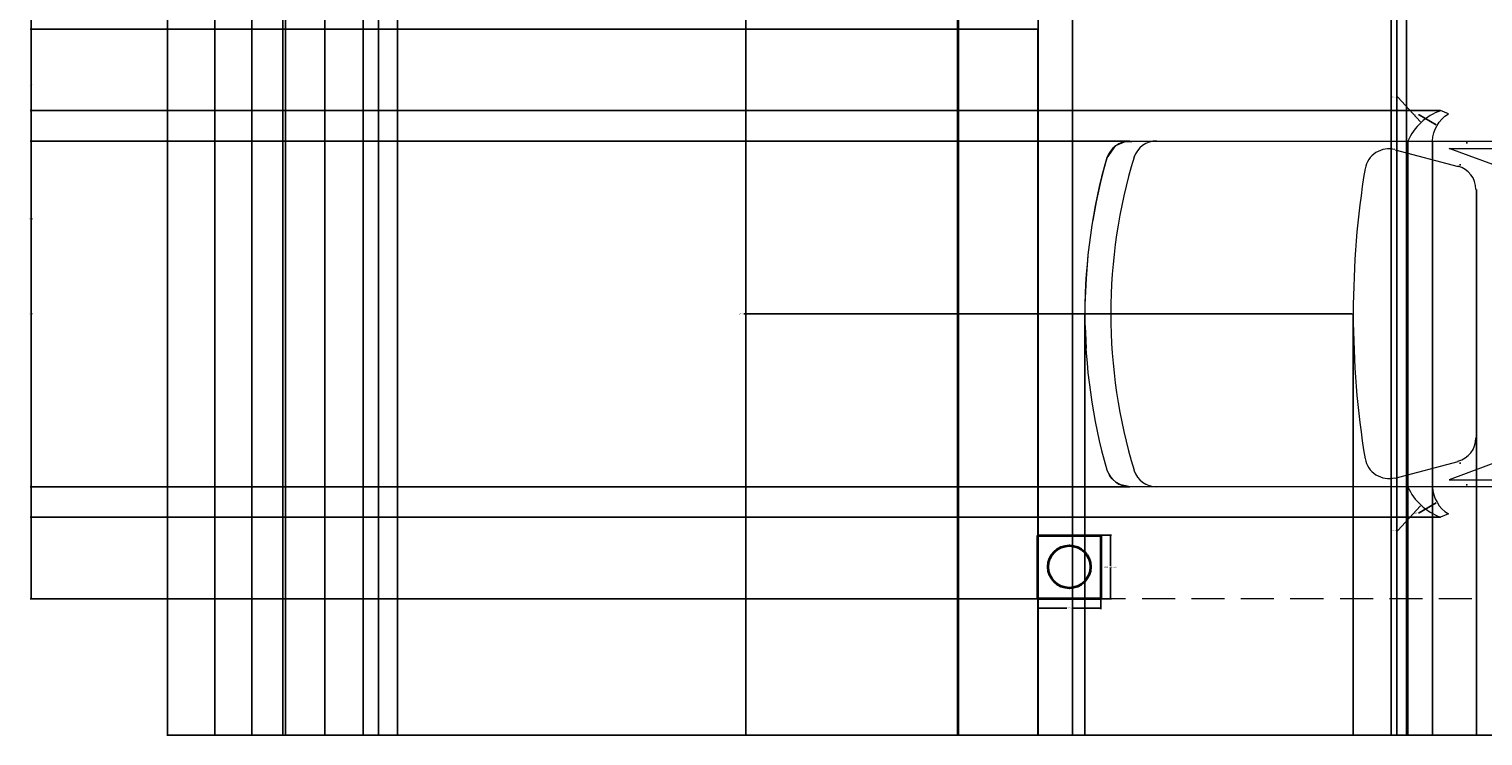
# Model space of a CAD drawing. Units: inches. Extents: x 6 to 575, y 34 to 566.
# Tile 1 of 21: x 6 to 282, y 34 to 168. Entities that reach past the tile are written whole.
import ezdxf

# ---------------------------------------------------------------- set-up
doc = ezdxf.new("R2010")
doc.units = ezdxf.units.IN
doc.linetypes.add('ACAD_ISO02W100', pattern=[15, 12, -3])
for name, color, linetype, lineweight in [('A-ANNO-DIMS', 2, 'Continuous', 18), ('A-COLS', 7, 'Continuous', 35), ('A-ROOF-OVHD', 240, 'ACAD_ISO02W100', 13), ('CARS', 5, 'Continuous', 18)]:
    doc.layers.add(name, color=color, linetype=linetype, lineweight=lineweight)
doc.styles.get("Standard").update_dxf_attribs({"font": 'arial.ttf'})
doc.dimstyles.get("Standard").update_dxf_attribs({"dimtxt": 0.18, "dimasz": 0.18, "dimexe": 0.18, "dimexo": 0.0625, "dimgap": 0.09, "dimtad": 0, "dimtih": 1, "dimtoh": 1, "dimdec": 4, "dimzin": 0, "dimdsep": 46, "dimtxsty": 'Standard', "dimcen": 0.09, "dimadec": 0, "dimazin": 0, "dimtfac": 1, "dimtdec": 4, "dimtofl": 0, "dimtmove": 0, "dimatfit": 3, "dimfxl": 1, "dimtolj": 1, "dimtzin": 0, "dimarcsym": 0})

# ---------------------------------------------------------------- blocks, each defined once
blk = doc.blocks.new('COL-PORTICO-RECT-BASE')
blk.add_lwpolyline([(0, 12.01), (11.94, 12.01), (11.94, 0), (0, 0)], close=True)
blk.add_circle((5.95, 6.05), 4.02)
blk = doc.blocks.new('*D23')
at = {"layer": 'A-ANNO-DIMS', "color": 0, "lineweight": -2, "transparency": 16777216}
for p, q in [((209.69, 71.79), (211.61, 71.79)), ((211.43, 71.61), (211.43, 65.97)), ((211.43, 59.96), (211.43, 65.6)), ((209.69, 59.78), (211.61, 59.78))]:
    blk.add_line(p, q, dxfattribs=at)
at = {"layer": 'A-ANNO-DIMS', "color": 0, "transparency": 16777216}
for points in [[(211.46, 71.61), (211.4, 71.61), (211.43, 71.79)], [(211.46, 59.96), (211.4, 59.96), (211.43, 59.78)]]:
    blk.add_solid(points, dxfattribs=at)
at = {"layer": 'Defpoints', "color": 0, "transparency": 16777216}
for p in [(209.62, 71.79), (211.43, 71.79), (209.62, 59.78)]:
    blk.add_point(p, dxfattribs=at)
at = {"layer": 'A-ANNO-DIMS', "color": 0, "transparency": 16777216, "insert": (211.43, 65.78), "char_height": 0.18, "attachment_point": 5}
blk.add_mtext('\\A1;COLUMN BASE L 12 TYP.', dxfattribs=at)
blk = doc.blocks.new('*D24')
at = {"layer": 'A-ANNO-DIMS', "color": 0, "lineweight": -2, "transparency": 16777216}
for p, q in [((197.69, 59.71), (197.69, 57.79)), ((197.87, 57.97), (203.14, 57.97)), ((209.44, 57.97), (204.18, 57.97)), ((209.62, 59.71), (209.62, 57.79))]:
    blk.add_line(p, q, dxfattribs=at)
at = {"layer": 'A-ANNO-DIMS', "color": 0, "transparency": 16777216}
for points in [[(197.87, 58), (197.87, 57.94), (197.69, 57.97)], [(209.44, 58), (209.44, 57.94), (209.62, 57.97)]]:
    blk.add_solid(points, dxfattribs=at)
at = {"layer": 'Defpoints', "color": 0, "transparency": 16777216}
for p in [(197.69, 59.77), (209.62, 59.78), (209.62, 57.97)]:
    blk.add_point(p, dxfattribs=at)
at = {"layer": 'A-ANNO-DIMS', "color": 0, "transparency": 16777216, "insert": (203.66, 57.97), "char_height": 0.18, "attachment_point": 5}
blk.add_mtext('\\A1;12 TYP.', dxfattribs=at)
blk = doc.blocks.new('*D29')
at = {"layer": 'A-ANNO-DIMS', "color": 0, "lineweight": -2, "transparency": 16777216}
for p, q in [((32.66, 203.74), (32.66, 33.76)), ((548.66, 203.74), (548.66, 33.76)), ((32.84, 33.94), (290.37, 33.94)), ((548.48, 33.94), (290.95, 33.94))]:
    blk.add_line(p, q, dxfattribs=at)
at = {"layer": 'A-ANNO-DIMS', "color": 0, "transparency": 16777216}
for points in [[(32.84, 33.97), (32.84, 33.91), (32.66, 33.94)], [(548.48, 33.97), (548.48, 33.91), (548.66, 33.94)]]:
    blk.add_solid(points, dxfattribs=at)
at = {"layer": 'Defpoints', "color": 0, "transparency": 16777216}
for p in [(32.66, 203.8), (548.66, 203.8), (548.66, 33.94)]:
    blk.add_point(p, dxfattribs=at)
at = {"layer": 'A-ANNO-DIMS', "color": 0, "transparency": 16777216, "insert": (290.66, 33.94), "char_height": 0.18, "attachment_point": 5}
blk.add_mtext('\\A1;516', dxfattribs=at)
blk = doc.blocks.new('*D30')
at = {"layer": 'A-ANNO-DIMS', "color": 0, "lineweight": -2, "transparency": 16777216}
for p, q in [((32.6, 539.8), (6.65, 539.8)), ((6.83, 539.62), (6.83, 299.97)), ((6.83, 59.95), (6.83, 299.61)), ((197.62, 59.77), (6.65, 59.77))]:
    blk.add_line(p, q, dxfattribs=at)
at = {"layer": 'A-ANNO-DIMS', "color": 0, "transparency": 16777216}
for points in [[(6.8, 539.62), (6.86, 539.62), (6.83, 539.8)], [(6.8, 59.95), (6.86, 59.95), (6.83, 59.77)]]:
    blk.add_solid(points, dxfattribs=at)
at = {"layer": 'Defpoints', "color": 0, "transparency": 16777216}
for p in [(32.66, 539.8), (6.83, 59.77), (197.69, 59.77)]:
    blk.add_point(p, dxfattribs=at)
at = {"layer": 'A-ANNO-DIMS', "color": 0, "transparency": 16777216, "insert": (6.83, 299.79), "char_height": 0.18, "attachment_point": 5}
blk.add_mtext('\\A1;480', dxfattribs=at)
blk = doc.blocks.new('*D48')
at = {"layer": 'A-ANNO-DIMS', "color": 0, "lineweight": -2, "transparency": 16777216}
for p, q in [((264.66, 215.74), (264.66, 33.76)), ((316.66, 215.74), (316.66, 33.76)), ((264.84, 33.94), (290.44, 33.94)), ((316.48, 33.94), (290.88, 33.94))]:
    blk.add_line(p, q, dxfattribs=at)
at = {"layer": 'A-ANNO-DIMS', "color": 0, "transparency": 16777216}
for points in [[(264.84, 33.97), (264.84, 33.91), (264.66, 33.94)], [(316.48, 33.97), (316.48, 33.91), (316.66, 33.94)]]:
    blk.add_solid(points, dxfattribs=at)
at = {"layer": 'Defpoints', "color": 0, "transparency": 16777216}
for p in [(264.66, 215.8), (316.66, 215.8), (316.66, 33.94)]:
    blk.add_point(p, dxfattribs=at)
at = {"layer": 'A-ANNO-DIMS', "color": 0, "transparency": 16777216, "insert": (290.66, 33.94), "char_height": 0.18, "attachment_point": 5}
blk.add_mtext('\\A1;52', dxfattribs=at)
blk = doc.blocks.new('*D76')
at = {"layer": 'A-ANNO-DIMS', "color": 0, "lineweight": -2, "transparency": 16777216}
for p, q in [((197.69, 59.71), (197.69, 33.76)), ((384.08, 59.71), (384.08, 33.76)), ((197.87, 33.94), (290.5, 33.94)), ((383.9, 33.94), (291.27, 33.94))]:
    blk.add_line(p, q, dxfattribs=at)
at = {"layer": 'A-ANNO-DIMS', "color": 0, "transparency": 16777216}
for points in [[(197.87, 33.97), (197.87, 33.91), (197.69, 33.94)], [(383.9, 33.97), (383.9, 33.91), (384.08, 33.94)]]:
    blk.add_solid(points, dxfattribs=at)
at = {"layer": 'Defpoints', "color": 0, "transparency": 16777216}
for p in [(197.69, 59.77), (384.08, 59.78), (384.08, 33.94)]:
    blk.add_point(p, dxfattribs=at)
at = {"layer": 'A-ANNO-DIMS', "color": 0, "transparency": 16777216, "insert": (290.88, 33.94), "char_height": 0.18, "attachment_point": 5}
blk.add_mtext('\\A1;186.4', dxfattribs=at)
blk = doc.blocks.new('*D77')
at = {"layer": 'A-ANNO-DIMS', "color": 0, "lineweight": -2, "transparency": 16777216}
for p, q in [((197.62, 203.8), (6.65, 203.8)), ((6.83, 203.62), (6.83, 131.97)), ((6.83, 59.95), (6.83, 131.61)), ((197.62, 59.77), (6.65, 59.77))]:
    blk.add_line(p, q, dxfattribs=at)
at = {"layer": 'A-ANNO-DIMS', "color": 0, "transparency": 16777216}
for points in [[(6.8, 203.62), (6.86, 203.62), (6.83, 203.8)], [(6.8, 59.95), (6.86, 59.95), (6.83, 59.77)]]:
    blk.add_solid(points, dxfattribs=at)
at = {"layer": 'Defpoints', "color": 0, "transparency": 16777216}
for p in [(6.83, 203.8), (197.69, 203.8), (197.69, 59.77)]:
    blk.add_point(p, dxfattribs=at)
at = {"layer": 'A-ANNO-DIMS', "color": 0, "transparency": 16777216, "insert": (6.83, 131.79), "char_height": 0.18, "attachment_point": 5}
blk.add_mtext('\\A1;144.03', dxfattribs=at)
blk = doc.blocks.new('*D78')
at = {"layer": 'A-ANNO-DIMS', "color": 0, "lineweight": -2, "transparency": 16777216}
for p, q in [((377.83, 117.84), (377.83, 33.76)), ((206.58, 113.74), (206.58, 33.76)), ((206.76, 33.94), (291.75, 33.94)), ((377.65, 33.94), (292.66, 33.94))]:
    blk.add_line(p, q, dxfattribs=at)
at = {"layer": 'A-ANNO-DIMS', "color": 0, "transparency": 16777216}
for points in [[(206.76, 33.97), (206.76, 33.91), (206.58, 33.94)], [(377.65, 33.97), (377.65, 33.91), (377.83, 33.94)]]:
    blk.add_solid(points, dxfattribs=at)
at = {"layer": 'Defpoints', "color": 0, "transparency": 16777216}
for p in [(377.83, 117.9), (206.58, 113.81), (377.83, 33.94)]:
    blk.add_point(p, dxfattribs=at)
at = {"layer": 'A-ANNO-DIMS', "color": 0, "transparency": 16777216, "insert": (292.21, 33.94), "char_height": 0.18, "attachment_point": 5}
blk.add_mtext('\\A1;171.25', dxfattribs=at)
blk = doc.blocks.new('*D79')
at = {"layer": 'A-ANNO-DIMS', "color": 0, "lineweight": -2, "transparency": 16777216}
for p, q in [((215.06, 146.53), (6.65, 146.53)), ((6.83, 146.35), (6.83, 113.95)), ((6.83, 81.18), (6.83, 113.58)), ((215.06, 81), (6.65, 81))]:
    blk.add_line(p, q, dxfattribs=at)
at = {"layer": 'A-ANNO-DIMS', "color": 0, "transparency": 16777216}
for points in [[(6.8, 146.35), (6.86, 146.35), (6.83, 146.53)], [(6.8, 81.18), (6.86, 81.18), (6.83, 81)]]:
    blk.add_solid(points, dxfattribs=at)
at = {"layer": 'Defpoints', "color": 0, "transparency": 16777216}
for p in [(6.83, 146.53), (215.12, 146.53), (215.12, 81)]:
    blk.add_point(p, dxfattribs=at)
at = {"layer": 'A-ANNO-DIMS', "color": 0, "transparency": 16777216, "insert": (6.83, 113.77), "char_height": 0.18, "attachment_point": 5}
blk.add_mtext('\\A1;65.54', dxfattribs=at)
blk = doc.blocks.new('*D80')
at = {"layer": 'A-ANNO-DIMS', "color": 0, "lineweight": -2, "transparency": 16777216}
for p, q in [((197.62, 167.76), (6.65, 167.76)), ((6.83, 167.58), (6.83, 157.33)), ((6.83, 146.71), (6.83, 156.96)), ((215.06, 146.53), (6.65, 146.53))]:
    blk.add_line(p, q, dxfattribs=at)
at = {"layer": 'A-ANNO-DIMS', "color": 0, "transparency": 16777216}
for points in [[(6.8, 167.58), (6.86, 167.58), (6.83, 167.76)], [(6.8, 146.71), (6.86, 146.71), (6.83, 146.53)]]:
    blk.add_solid(points, dxfattribs=at)
at = {"layer": 'Defpoints', "color": 0, "transparency": 16777216}
for p in [(6.83, 167.76), (197.69, 167.76), (215.12, 146.53)]:
    blk.add_point(p, dxfattribs=at)
at = {"layer": 'A-ANNO-DIMS', "color": 0, "transparency": 16777216, "insert": (6.83, 157.15), "char_height": 0.18, "attachment_point": 5}
blk.add_mtext('\\A1;21.22', dxfattribs=at)
blk = doc.blocks.new('*D81')
at = {"layer": 'A-ANNO-DIMS', "color": 0, "lineweight": -2, "transparency": 16777216}
for p, q in [((280.78, 137.27), (280.78, 33.76)), ((257.45, 113.74), (257.45, 33.76)), ((257.63, 33.94), (268.72, 33.94)), ((280.6, 33.94), (269.51, 33.94))]:
    blk.add_line(p, q, dxfattribs=at)
at = {"layer": 'A-ANNO-DIMS', "color": 0, "transparency": 16777216}
for points in [[(257.63, 33.97), (257.63, 33.91), (257.45, 33.94)], [(280.6, 33.97), (280.6, 33.91), (280.78, 33.94)]]:
    blk.add_solid(points, dxfattribs=at)
at = {"layer": 'Defpoints', "color": 0, "transparency": 16777216}
for p in [(280.78, 137.33), (257.45, 113.81), (280.78, 33.94)]:
    blk.add_point(p, dxfattribs=at)
at = {"layer": 'A-ANNO-DIMS', "color": 0, "transparency": 16777216, "insert": (269.11, 33.94), "char_height": 0.18, "attachment_point": 5}
blk.add_mtext('\\A1;23.33', dxfattribs=at)
blk = doc.blocks.new('*D83')
at = {"layer": 'A-ANNO-DIMS', "color": 0, "lineweight": -2, "transparency": 16777216}
for p, q in [((197.69, 167.69), (197.69, 33.76)), ((206.58, 113.74), (206.58, 33.76)), ((197.87, 33.94), (201.74, 33.94)), ((206.4, 33.94), (202.53, 33.94))]:
    blk.add_line(p, q, dxfattribs=at)
at = {"layer": 'A-ANNO-DIMS', "color": 0, "transparency": 16777216}
for points in [[(197.87, 33.97), (197.87, 33.91), (197.69, 33.94)], [(206.4, 33.97), (206.4, 33.91), (206.58, 33.94)]]:
    blk.add_solid(points, dxfattribs=at)
at = {"layer": 'Defpoints', "color": 0, "transparency": 16777216}
for p in [(197.69, 167.76), (206.58, 113.81), (206.58, 33.94)]:
    blk.add_point(p, dxfattribs=at)
at = {"layer": 'A-ANNO-DIMS', "color": 0, "transparency": 16777216, "insert": (202.13, 33.94), "char_height": 0.18, "attachment_point": 5}
blk.add_mtext('\\A1;8.894', dxfattribs=at)
blk = doc.blocks.new('*D84')
at = {"layer": 'A-ANNO-DIMS', "color": 0, "lineweight": -2, "transparency": 16777216}
for p, q in [((206.58, 113.74), (206.58, 33.76)), ((257.45, 113.74), (257.45, 33.76)), ((206.76, 33.94), (231.62, 33.94)), ((257.27, 33.94), (232.41, 33.94))]:
    blk.add_line(p, q, dxfattribs=at)
at = {"layer": 'A-ANNO-DIMS', "color": 0, "transparency": 16777216}
for points in [[(206.76, 33.97), (206.76, 33.91), (206.58, 33.94)], [(257.27, 33.97), (257.27, 33.91), (257.45, 33.94)]]:
    blk.add_solid(points, dxfattribs=at)
at = {"layer": 'Defpoints', "color": 0, "transparency": 16777216}
for p in [(206.58, 113.81), (257.45, 113.81), (257.45, 33.94)]:
    blk.add_point(p, dxfattribs=at)
at = {"layer": 'A-ANNO-DIMS', "color": 0, "transparency": 16777216, "insert": (232.02, 33.94), "char_height": 0.18, "attachment_point": 5}
blk.add_mtext('\\A1;50.87', dxfattribs=at)
blk = doc.blocks.new('*D85')
at = {"layer": 'A-ANNO-DIMS', "color": 0, "lineweight": -2, "transparency": 16777216}
for p, q in [((338.19, 140.75), (338.19, 33.76)), ((280.78, 137.27), (280.78, 33.76)), ((280.96, 33.94), (309.11, 33.94)), ((338.01, 33.94), (309.86, 33.94))]:
    blk.add_line(p, q, dxfattribs=at)
at = {"layer": 'A-ANNO-DIMS', "color": 0, "transparency": 16777216}
for points in [[(280.96, 33.97), (280.96, 33.91), (280.78, 33.94)], [(338.01, 33.97), (338.01, 33.91), (338.19, 33.94)]]:
    blk.add_solid(points, dxfattribs=at)
at = {"layer": 'Defpoints', "color": 0, "transparency": 16777216}
for p in [(338.19, 140.81), (280.78, 137.33), (338.19, 33.94)]:
    blk.add_point(p, dxfattribs=at)
at = {"layer": 'A-ANNO-DIMS', "color": 0, "transparency": 16777216, "insert": (309.48, 33.94), "char_height": 0.18, "attachment_point": 5}
blk.add_mtext('\\A1;57.41', dxfattribs=at)
blk = doc.blocks.new('*D87')
at = {"layer": 'A-ANNO-DIMS', "color": 0, "lineweight": -2, "transparency": 16777216}
for p, q in [((273.93, 152.31), (6.65, 152.31)), ((6.83, 152.13), (6.83, 113.96)), ((6.83, 75.42), (6.83, 113.59)), ((273.95, 75.24), (6.65, 75.24))]:
    blk.add_line(p, q, dxfattribs=at)
at = {"layer": 'A-ANNO-DIMS', "color": 0, "transparency": 16777216}
for points in [[(6.8, 152.13), (6.86, 152.13), (6.83, 152.31)], [(6.8, 75.42), (6.86, 75.42), (6.83, 75.24)]]:
    blk.add_solid(points, dxfattribs=at)
at = {"layer": 'Defpoints', "color": 0, "transparency": 16777216}
for p in [(273.99, 152.31), (6.83, 75.24), (274.01, 75.24)]:
    blk.add_point(p, dxfattribs=at)
at = {"layer": 'A-ANNO-DIMS', "color": 0, "transparency": 16777216, "insert": (6.83, 113.78), "char_height": 0.18, "attachment_point": 5}
blk.add_mtext('\\A1;77.06', dxfattribs=at)
blk = doc.blocks.new('*D88')
at = {"layer": 'A-ANNO-DIMS', "color": 0, "lineweight": -2, "transparency": 16777216}
for p, q in [((267.78, 146.47), (267.78, 33.76)), ((272.44, 146.49), (272.44, 33.76)), ((267.96, 33.94), (269.71, 33.94)), ((272.26, 33.94), (270.51, 33.94))]:
    blk.add_line(p, q, dxfattribs=at)
at = {"layer": 'A-ANNO-DIMS', "color": 0, "transparency": 16777216}
for points in [[(267.96, 33.97), (267.96, 33.91), (267.78, 33.94)], [(272.26, 33.97), (272.26, 33.91), (272.44, 33.94)]]:
    blk.add_solid(points, dxfattribs=at)
at = {"layer": 'Defpoints', "color": 0, "transparency": 16777216}
for p in [(267.78, 146.54), (272.44, 146.55), (272.44, 33.94)]:
    blk.add_point(p, dxfattribs=at)
at = {"layer": 'A-ANNO-DIMS', "color": 0, "transparency": 16777216, "insert": (270.11, 33.94), "char_height": 0.18, "attachment_point": 5}
blk.add_mtext('\\A1;4.659', dxfattribs=at)
blk = doc.blocks.new('*D89')
at = {"layer": 'A-ANNO-DIMS', "color": 0, "lineweight": -2, "transparency": 16777216}
for p, q in [((267.78, 146.47), (267.78, 33.76)), ((257.45, 113.74), (257.45, 33.76)), ((257.63, 33.94), (262.18, 33.94)), ((267.6, 33.94), (263.05, 33.94))]:
    blk.add_line(p, q, dxfattribs=at)
at = {"layer": 'A-ANNO-DIMS', "color": 0, "transparency": 16777216}
for points in [[(257.63, 33.97), (257.63, 33.91), (257.45, 33.94)], [(267.6, 33.97), (267.6, 33.91), (267.78, 33.94)]]:
    blk.add_solid(points, dxfattribs=at)
at = {"layer": 'Defpoints', "color": 0, "transparency": 16777216}
for p in [(267.78, 146.54), (257.45, 113.81), (257.45, 33.94)]:
    blk.add_point(p, dxfattribs=at)
at = {"layer": 'A-ANNO-DIMS', "color": 0, "transparency": 16777216, "insert": (262.61, 33.94), "char_height": 0.18, "attachment_point": 5}
blk.add_mtext('\\A1;10.331', dxfattribs=at)
blk = doc.blocks.new('*D91')
at = {"layer": 'A-ANNO-DIMS', "color": 0, "lineweight": -2, "transparency": 16777216}
for p, q in [((62.49, 286), (62.49, 33.76)), ((41.66, 265.01), (41.66, 33.76)), ((41.84, 33.94), (51.68, 33.94)), ((62.31, 33.94), (52.47, 33.94))]:
    blk.add_line(p, q, dxfattribs=at)
at = {"layer": 'A-ANNO-DIMS', "color": 0, "transparency": 16777216}
for points in [[(41.84, 33.97), (41.84, 33.91), (41.66, 33.94)], [(62.31, 33.97), (62.31, 33.91), (62.49, 33.94)]]:
    blk.add_solid(points, dxfattribs=at)
at = {"layer": 'Defpoints', "color": 0, "transparency": 16777216}
for p in [(62.49, 286.06), (41.66, 265.08), (62.49, 33.94)]:
    blk.add_point(p, dxfattribs=at)
at = {"layer": 'A-ANNO-DIMS', "color": 0, "transparency": 16777216, "insert": (52.07, 33.94), "char_height": 0.18, "attachment_point": 5}
blk.add_mtext('\\A1;20.83', dxfattribs=at)
blk = doc.blocks.new('*D93')
at = {"layer": 'A-ANNO-DIMS', "color": 0, "lineweight": -2, "transparency": 16777216}
for p, q in [((54.53, 298.17), (54.53, 33.76)), ((69.75, 298.17), (69.75, 33.76)), ((54.71, 33.94), (61.68, 33.94)), ((69.57, 33.94), (62.59, 33.94))]:
    blk.add_line(p, q, dxfattribs=at)
at = {"layer": 'A-ANNO-DIMS', "color": 0, "transparency": 16777216}
for points in [[(54.71, 33.97), (54.71, 33.91), (54.53, 33.94)], [(69.57, 33.97), (69.57, 33.91), (69.75, 33.94)]]:
    blk.add_solid(points, dxfattribs=at)
at = {"layer": 'Defpoints', "color": 0, "transparency": 16777216}
for p in [(54.53, 298.24), (69.75, 298.24), (69.75, 33.94)]:
    blk.add_point(p, dxfattribs=at)
at = {"layer": 'A-ANNO-DIMS', "color": 0, "transparency": 16777216, "insert": (62.14, 33.94), "char_height": 0.18, "attachment_point": 5}
blk.add_mtext('\\A1;15.214', dxfattribs=at)
blk = doc.blocks.new('*D97')
at = {"layer": 'A-ANNO-DIMS', "color": 0, "lineweight": -2, "transparency": 16777216}
for p, q in [((55.08, 297.86), (55.08, 33.76)), ((41.66, 286), (41.66, 33.76)), ((41.84, 33.94), (47.98, 33.94)), ((54.9, 33.94), (48.75, 33.94))]:
    blk.add_line(p, q, dxfattribs=at)
at = {"layer": 'A-ANNO-DIMS', "color": 0, "transparency": 16777216}
for points in [[(41.84, 33.97), (41.84, 33.91), (41.66, 33.94)], [(54.9, 33.97), (54.9, 33.91), (55.08, 33.94)]]:
    blk.add_solid(points, dxfattribs=at)
at = {"layer": 'Defpoints', "color": 0, "transparency": 16777216}
for p in [(55.08, 297.92), (41.66, 286.06), (55.08, 33.94)]:
    blk.add_point(p, dxfattribs=at)
at = {"layer": 'A-ANNO-DIMS', "color": 0, "transparency": 16777216, "insert": (48.37, 33.94), "char_height": 0.18, "attachment_point": 5}
blk.add_mtext('\\A1;13.42', dxfattribs=at)
blk = doc.blocks.new('*D98')
at = {"layer": 'A-ANNO-DIMS', "color": 0, "lineweight": -2, "transparency": 16777216}
for p, q in [((48.68, 220.31), (48.68, 33.76)), ((41.66, 212.74), (41.66, 33.76)), ((41.84, 33.94), (44.78, 33.94)), ((48.5, 33.94), (45.56, 33.94))]:
    blk.add_line(p, q, dxfattribs=at)
at = {"layer": 'A-ANNO-DIMS', "color": 0, "transparency": 16777216}
for points in [[(41.84, 33.97), (41.84, 33.91), (41.66, 33.94)], [(48.5, 33.97), (48.5, 33.91), (48.68, 33.94)]]:
    blk.add_solid(points, dxfattribs=at)
at = {"layer": 'Defpoints', "color": 0, "transparency": 16777216}
for p in [(48.68, 220.37), (41.66, 212.8), (48.68, 33.94)]:
    blk.add_point(p, dxfattribs=at)
at = {"layer": 'A-ANNO-DIMS', "color": 0, "transparency": 16777216, "insert": (45.17, 33.94), "char_height": 0.18, "attachment_point": 5}
blk.add_mtext('\\A1;7.022', dxfattribs=at)
blk = doc.blocks.new('*D100')
at = {"layer": 'A-ANNO-DIMS', "color": 0, "lineweight": -2, "transparency": 16777216}
for p, q in [((76.3, 221.52), (76.3, 33.76)), ((72.71, 220.31), (72.71, 33.76)), ((72.89, 33.94), (74.11, 33.94)), ((76.12, 33.94), (74.9, 33.94))]:
    blk.add_line(p, q, dxfattribs=at)
at = {"layer": 'A-ANNO-DIMS', "color": 0, "transparency": 16777216}
for points in [[(72.89, 33.97), (72.89, 33.91), (72.71, 33.94)], [(76.12, 33.97), (76.12, 33.91), (76.3, 33.94)]]:
    blk.add_solid(points, dxfattribs=at)
at = {"layer": 'Defpoints', "color": 0, "transparency": 16777216}
for p in [(76.3, 221.58), (72.71, 220.37), (76.3, 33.94)]:
    blk.add_point(p, dxfattribs=at)
at = {"layer": 'A-ANNO-DIMS', "color": 0, "transparency": 16777216, "insert": (74.5, 33.94), "char_height": 0.18, "attachment_point": 5}
blk.add_mtext('\\A1;3.589', dxfattribs=at)
blk = doc.blocks.new('*D101')
at = {"layer": 'A-ANNO-DIMS', "color": 0, "lineweight": -2, "transparency": 16777216}
for p, q in [((76.3, 221.52), (76.3, 33.76)), ((142.3, 221.48), (142.3, 33.76)), ((76.48, 33.94), (109.08, 33.94)), ((142.12, 33.94), (109.52, 33.94))]:
    blk.add_line(p, q, dxfattribs=at)
at = {"layer": 'A-ANNO-DIMS', "color": 0, "transparency": 16777216}
for points in [[(76.48, 33.97), (76.48, 33.91), (76.3, 33.94)], [(142.12, 33.97), (142.12, 33.91), (142.3, 33.94)]]:
    blk.add_solid(points, dxfattribs=at)
at = {"layer": 'Defpoints', "color": 0, "transparency": 16777216}
for p in [(76.3, 221.58), (142.3, 221.54), (142.3, 33.94)]:
    blk.add_point(p, dxfattribs=at)
at = {"layer": 'A-ANNO-DIMS', "color": 0, "transparency": 16777216, "insert": (109.3, 33.94), "char_height": 0.18, "attachment_point": 5}
blk.add_mtext('\\A1;66', dxfattribs=at)
blk = doc.blocks.new('*D105')
at = {"layer": 'A-ANNO-DIMS', "color": 0, "lineweight": -2, "transparency": 16777216}
for p, q in [((182.64, 293.1), (182.64, 33.76)), ((197.7, 293.1), (197.7, 33.76)), ((182.82, 33.94), (189.71, 33.94)), ((197.52, 33.94), (190.62, 33.94))]:
    blk.add_line(p, q, dxfattribs=at)
at = {"layer": 'A-ANNO-DIMS', "color": 0, "transparency": 16777216}
for points in [[(182.82, 33.97), (182.82, 33.91), (182.64, 33.94)], [(197.52, 33.97), (197.52, 33.91), (197.7, 33.94)]]:
    blk.add_solid(points, dxfattribs=at)
at = {"layer": 'Defpoints', "color": 0, "transparency": 16777216}
for p in [(182.64, 293.16), (197.7, 293.16), (197.7, 33.94)]:
    blk.add_point(p, dxfattribs=at)
at = {"layer": 'A-ANNO-DIMS', "color": 0, "transparency": 16777216, "insert": (190.17, 33.94), "char_height": 0.18, "attachment_point": 5}
blk.add_mtext('\\A1;15.058', dxfattribs=at)
blk = doc.blocks.new('*D208')
at = {"layer": 'A-ANNO-DIMS', "color": 0, "lineweight": -2, "transparency": 16777216}
for p, q in [((182.44, 270.6), (182.44, 33.76)), ((204.24, 232.86), (204.24, 33.76)), ((182.62, 33.94), (192.88, 33.94)), ((204.06, 33.94), (193.81, 33.94))]:
    blk.add_line(p, q, dxfattribs=at)
at = {"layer": 'A-ANNO-DIMS', "color": 0, "transparency": 16777216}
for points in [[(182.62, 33.97), (182.62, 33.91), (182.44, 33.94)], [(204.06, 33.97), (204.06, 33.91), (204.24, 33.94)]]:
    blk.add_solid(points, dxfattribs=at)
at = {"layer": 'Defpoints', "color": 0, "transparency": 16777216}
for p in [(182.44, 270.67), (204.24, 232.92), (182.44, 33.94)]:
    blk.add_point(p, dxfattribs=at)
at = {"layer": 'A-ANNO-DIMS', "color": 0, "transparency": 16777216, "insert": (193.34, 33.94), "char_height": 0.18, "attachment_point": 5}
blk.add_mtext('\\A1;21.793', dxfattribs=at)
blk = doc.blocks.new('*D210')
at = {"layer": 'A-ANNO-DIMS', "color": 0, "lineweight": -2, "transparency": 16777216}
for p, q in [((265.7, 249.02), (265.7, 33.76)), ((267.52, 249.02), (267.52, 33.76)), ((265.88, 33.94), (266.29, 33.94)), ((267.34, 33.94), (266.92, 33.94))]:
    blk.add_line(p, q, dxfattribs=at)
at = {"layer": 'A-ANNO-DIMS', "color": 0, "transparency": 16777216}
for points in [[(265.88, 33.97), (265.88, 33.91), (265.7, 33.94)], [(267.34, 33.97), (267.34, 33.91), (267.52, 33.94)]]:
    blk.add_solid(points, dxfattribs=at)
at = {"layer": 'Defpoints', "color": 0, "transparency": 16777216}
for p in [(265.7, 249.08), (267.52, 249.08), (267.52, 33.94)]:
    blk.add_point(p, dxfattribs=at)
at = {"layer": 'A-ANNO-DIMS', "color": 0, "transparency": 16777216, "insert": (266.61, 33.94), "char_height": 0.18, "attachment_point": 5}
blk.add_mtext('\\A1;1.82', dxfattribs=at)
blk = doc.blocks.new('*D220')
at = {"layer": 'A-ANNO-DIMS', "color": 0, "lineweight": -2, "transparency": 16777216}
for p, q in [((155, 113.8), (257.27, 113.8)), ((428.11, 113.81), (428.29, 113.81)), ((428.2, 113.72), (428.2, 113.9))]:
    blk.add_line(p, q, dxfattribs=at)
at = {"layer": 'A-ANNO-DIMS', "color": 0, "transparency": 16777216}
blk.add_solid([(257.27, 113.83), (257.27, 113.77), (257.45, 113.8)], dxfattribs=at)
at = {"layer": 'Defpoints', "color": 0, "transparency": 16777216}
for p in [(257.45, 113.8), (428.2, 113.81)]:
    blk.add_point(p, dxfattribs=at)
at = {"layer": 'A-ANNO-DIMS', "color": 0, "transparency": 16777216, "insert": (154.45, 113.8), "char_height": 0.18, "attachment_point": 5}
blk.add_mtext('\\A1;R170.75', dxfattribs=at)
blk = doc.blocks.new('*D221')
at = {"layer": 'A-ANNO-DIMS', "color": 0, "lineweight": -2, "transparency": 16777216}
for p, q in [((141.91, 113.8), (206.4, 113.8)), ((314.28, 113.81), (314.46, 113.81)), ((314.37, 113.72), (314.37, 113.9))]:
    blk.add_line(p, q, dxfattribs=at)
at = {"layer": 'A-ANNO-DIMS', "color": 0, "transparency": 16777216}
blk.add_solid([(206.4, 113.83), (206.4, 113.77), (206.58, 113.8)], dxfattribs=at)
at = {"layer": 'Defpoints', "color": 0, "transparency": 16777216}
for p in [(206.58, 113.8), (314.37, 113.81)]:
    blk.add_point(p, dxfattribs=at)
at = {"layer": 'A-ANNO-DIMS', "color": 0, "transparency": 16777216, "insert": (141.36, 113.8), "char_height": 0.18, "attachment_point": 5}
blk.add_mtext('\\A1;R107.78', dxfattribs=at)
blk = doc.blocks.new('*D222')
at = {"layer": 'A-ANNO-DIMS', "color": 0, "lineweight": -2, "transparency": 16777216}
for p, q in [((150.38, 113.8), (211.32, 113.8)), ((313.26, 113.81), (313.44, 113.81)), ((313.35, 113.72), (313.35, 113.9))]:
    blk.add_line(p, q, dxfattribs=at)
at = {"layer": 'A-ANNO-DIMS', "color": 0, "transparency": 16777216}
blk.add_solid([(211.32, 113.83), (211.32, 113.77), (211.5, 113.8)], dxfattribs=at)
at = {"layer": 'Defpoints', "color": 0, "transparency": 16777216}
for p in [(211.5, 113.8), (313.35, 113.81)]:
    blk.add_point(p, dxfattribs=at)
at = {"layer": 'A-ANNO-DIMS', "color": 0, "transparency": 16777216, "insert": (149.83, 113.8), "char_height": 0.18, "attachment_point": 5}
blk.add_mtext('\\A1;R101.85', dxfattribs=at)
blk = doc.blocks.new('*D236')
at = {"layer": 'A-ANNO-DIMS', "color": 0, "lineweight": -2, "transparency": 16777216}
for p, q in [((277.61, 85.48), (277.79, 85.48)), ((277.7, 85.39), (277.7, 85.57)), ((265.88, 72.69), (270.19, 77.36)), ((265.7, 72.69), (265.88, 72.69))]:
    blk.add_line(p, q, dxfattribs=at)
at = {"layer": 'A-ANNO-DIMS', "color": 0, "transparency": 16777216}
blk.add_solid([(270.17, 77.38), (270.21, 77.34), (270.31, 77.49)], dxfattribs=at)
at = {"layer": 'Defpoints', "color": 0, "transparency": 16777216}
for p in [(277.7, 85.48), (270.31, 77.49)]:
    blk.add_point(p, dxfattribs=at)
at = {"layer": 'A-ANNO-DIMS', "color": 0, "transparency": 16777216, "insert": (265.15, 72.69), "char_height": 0.18, "attachment_point": 5}
blk.add_mtext('\\A1;R10.884', dxfattribs=at)
blk = doc.blocks.new('*D237')
at = {"layer": 'A-ANNO-DIMS', "color": 0, "lineweight": -2, "transparency": 16777216}
for p, q in [((265.7, 154.84), (265.88, 154.84)), ((265.88, 154.84), (270.19, 150.18)), ((277.61, 142.05), (277.79, 142.05)), ((277.7, 141.96), (277.7, 142.14))]:
    blk.add_line(p, q, dxfattribs=at)
at = {"layer": 'A-ANNO-DIMS', "color": 0, "transparency": 16777216}
blk.add_solid([(270.21, 150.2), (270.17, 150.16), (270.31, 150.04)], dxfattribs=at)
at = {"layer": 'Defpoints', "color": 0, "transparency": 16777216}
for p in [(270.31, 150.04), (277.7, 142.05)]:
    blk.add_point(p, dxfattribs=at)
at = {"layer": 'A-ANNO-DIMS', "color": 0, "transparency": 16777216, "insert": (265.15, 154.84), "char_height": 0.18, "attachment_point": 5}
blk.add_mtext('\\A1;R10.884', dxfattribs=at)
blk = doc.blocks.new('*D241')
at = {"layer": 'A-ANNO-DIMS', "color": 0, "lineweight": -2, "transparency": 16777216}
for p, q in [((269.79, 151.47), (269.97, 151.47)), ((269.97, 151.47), (273.18, 149.58)), ((278.86, 146.17), (279.04, 146.17)), ((278.95, 146.08), (278.95, 146.26))]:
    blk.add_line(p, q, dxfattribs=at)
at = {"layer": 'A-ANNO-DIMS', "color": 0, "transparency": 16777216}
blk.add_solid([(273.19, 149.6), (273.16, 149.55), (273.33, 149.48)], dxfattribs=at)
at = {"layer": 'Defpoints', "color": 0, "transparency": 16777216}
for p in [(273.33, 149.48), (278.95, 146.17)]:
    blk.add_point(p, dxfattribs=at)
at = {"layer": 'A-ANNO-DIMS', "color": 0, "transparency": 16777216, "insert": (269.38, 151.47), "char_height": 0.18, "attachment_point": 5}
blk.add_mtext('\\A1;R6.52', dxfattribs=at)
blk = doc.blocks.new('*D242')
at = {"layer": 'A-ANNO-DIMS', "color": 0, "lineweight": -2, "transparency": 16777216}
for p, q in [((278.86, 81.36), (279.04, 81.36)), ((278.95, 81.27), (278.95, 81.45)), ((269.97, 76.06), (273.18, 77.96)), ((269.79, 76.06), (269.97, 76.06))]:
    blk.add_line(p, q, dxfattribs=at)
at = {"layer": 'A-ANNO-DIMS', "color": 0, "transparency": 16777216}
blk.add_solid([(273.16, 77.98), (273.19, 77.93), (273.33, 78.05)], dxfattribs=at)
at = {"layer": 'Defpoints', "color": 0, "transparency": 16777216}
for p in [(278.95, 81.36), (273.33, 78.05)]:
    blk.add_point(p, dxfattribs=at)
at = {"layer": 'A-ANNO-DIMS', "color": 0, "transparency": 16777216, "insert": (269.31, 76.06), "char_height": 0.18, "attachment_point": 5}
blk.add_mtext('\\A1;R6.519', dxfattribs=at)

msp = doc.modelspace()

# ---------------------------------------------------------------- linework, layer by layer
at = {"layer": 'A-ROOF-OVHD'}
for points in [[(197.6864, 161.4363), (197.6864, 167.6779)], [(197.6864, 152.074), (197.6864, 158.3155)], [(197.6864, 142.7116), (197.6864, 148.9532)], [(197.6864, 133.3493), (197.6864, 139.5908)], [(197.6864, 123.9869), (197.6864, 130.2285)], [(197.6864, 114.5465), (197.6864, 120.8661)], [(197.6864, 105.1842), (197.6864, 111.4257)], [(197.6864, 95.8218), (197.6864, 102.0634)], [(197.6864, 86.4595), (197.6864, 92.701)], [(197.6864, 77.0971), (197.6864, 83.3387)], [(197.6864, 67.7348), (197.6864, 73.9763)], [(204.9422, 59.7768), (197.6864, 59.7768), (197.6864, 64.614)], [(214.3046, 59.7768), (208.063, 59.7768)], [(223.6669, 59.7768), (217.4254, 59.7768)], [(233.0293, 59.7768), (226.7877, 59.7768)], [(242.3916, 59.7768), (236.1501, 59.7768)], [(251.832, 59.7768), (245.5124, 59.7768)], [(261.1944, 59.7768), (254.9528, 59.7768)], [(270.5567, 59.7768), (264.3151, 59.7768)], [(279.9191, 59.7768), (273.6775, 59.7768)]]:
    msp.add_lwpolyline(points, dxfattribs=at)
at = {"layer": 'CARS'}
for points in [[(272.4396, 146.5506, -0.24202223), (275.472, 151.6839), (273.9896, 152.308)], [(272.4396, 80.9821, 0.24202253), (275.472, 75.8488), (273.9896, 75.2246)]]:
    msp.add_lwpolyline(points, format="xyb", dxfattribs=at)
for points in [[(208.141, 131.4768), (208.7652, 134.9877), (209.5454, 138.4986), (210.2475, 141.3073), (210.7937, 143.3358), (212.4321, 145.6764), (214.0705, 146.3785), (216.9572, 146.5346)], [(215.1628, 146.5346), (371.6702, 146.5346)], [(265.4074, 144.8962), (277.3444, 141.6974)], [(280.7773, 137.3283), (280.7773, 90.2044)], [(206.8927, 107.2127), (206.7367, 110.2555), (206.6586, 112.0499), (206.6586, 115.5608), (206.8927, 120.476), (207.2048, 124.7671)], [(265.4074, 82.6365), (277.3444, 85.7573)], [(371.5921, 80.9981), (215.1628, 80.9981), (213.3683, 81.3882), (212.4321, 81.8563), (211.7299, 82.4805), (211.2618, 83.1046)]]:
    msp.add_lwpolyline(points, dxfattribs=at)
for points in [[(316.5883, 145.1302), (316.5883, 141.3853), (285.7705, 141.3853), (275.628, 145.1302)], [(275.628, 82.3244), (316.5883, 82.3244), (316.5883, 86.0694), (285.7705, 86.0694)]]:
    msp.add_lwpolyline(points, close=True, dxfattribs=at)
for centre, radius, start, end in [((277.6955, 142.0484), 10.8837, 109.791852, 155.643282), ((215.1238, 141.9705), 4.5641, 89.999915, 162.548422), ((220.1951, 141.9704), 4.5641, 90.000056, 161.466065), ((314.3651, 113.8053), 107.7845, 164.069878, 195.930122), ((313.3508, 113.8053), 101.8549, 163.070118, 196.929882), ((264.1981, 140.488), 4.5642, 75.256368, 170.06201), ((428.196, 113.8053), 170.7466, 170.733066, 189.266934), ((276.1351, 137.3673), 4.5641, 359.999899, 75.256131), ((276.1351, 90.2434), 4.5641, 284.743829, 0.000141), ((264.1982, 87.1227), 4.5643, 189.938033, 284.743605), ((215.1238, 85.5622), 4.5641, 197.451633, 270.00003), ((220.1951, 85.5622), 4.5641, 198.533798, 269.999998), ((277.6955, 85.4843), 10.8838, 204.356786, 250.208078)]:
    msp.add_arc(centre, radius, start, end, dxfattribs=at)

# ---------------------------------------------------------------- block references
at = {"layer": 'A-COLS', "rotation": 0.0063871507236521}
msp.add_blockref('COL-PORTICO-RECT-BASE', (197.6868, 59.7747), dxfattribs=at)

# ---------------------------------------------------------------- dimensions: what is measured, and where the dimension line sits
at = {"layer": 'A-ANNO-DIMS'}
for base, p1, p2, override, picture, middle in [((6.8286, 59.7747), (32.6586, 539.801), (197.6872, 59.7747), {"dimdec": 0, "dimlfac": 1, "dimrnd": 0, "dimzin": 0, "dimdsep": 46, "dimlunit": 2}, '*D30', (6.8286, 299.7878)), ((6.8286, 203.801), (197.6872, 59.7747), (197.6864, 203.801), {"dimdec": 2, "dimlfac": 1, "dimrnd": 0, "dimzin": 0, "dimdsep": 46, "dimlunit": 2}, '*D77', (6.8286, 131.7878)), ((6.8286, 167.7559), (215.1238, 146.5346), (197.6864, 167.7559), {"dimdec": 2, "dimlfac": 1, "dimrnd": 0, "dimzin": 0, "dimdsep": 46, "dimlunit": 2}, '*D80', (6.8286, 157.1452)), ((6.8286, 75.2434), (273.9896, 152.308), (274.0102, 75.2434), {"dimdec": 2, "dimlfac": 1, "dimrnd": 0, "dimzin": 0, "dimdsep": 46, "dimlunit": 2}, '*D87', (6.8286, 113.7757)), ((6.8286, 146.5346), (215.1238, 80.9981), (215.1238, 146.5346), {"dimdec": 2, "dimlfac": 1, "dimrnd": 0, "dimzin": 0, "dimdsep": 46, "dimlunit": 2}, '*D79', (6.8286, 113.7663))]:
    dim = msp.add_linear_dim(base=base, p1=p1, p2=p2, angle=90, dimstyle='Standard', override=override, dxfattribs=at)
    dim.commit()
    dim.dimension.update_dxf_attribs({"geometry": picture, "text_midpoint": middle})
for base, p1, p2, override, picture, middle in [((55.078, 33.9447), (41.6586, 286.0643), (55.078, 297.9233), {"dimdec": 2, "dimlfac": 1, "dimrnd": 0, "dimzin": 0, "dimdsep": 46, "dimlunit": 2}, '*D97', (48.3683, 33.9447)), ((69.7457, 33.9447), (54.5319, 298.2354), (69.7457, 298.2354), {"dimdec": 3, "dimlfac": 1, "dimrnd": 0, "dimzin": 0, "dimdsep": 46, "dimlunit": 2}, '*D93', (62.1388, 33.9447)), ((197.6979, 33.9447), (182.6401, 293.1641), (197.6979, 293.1641), {"dimdec": 3, "dimlfac": 1, "dimrnd": 0, "dimzin": 0, "dimdsep": 46, "dimlunit": 2}, '*D105', (190.169, 33.9447)), ((62.4899, 33.9447), (41.6586, 265.077), (62.4899, 286.0643), {"dimdec": 2, "dimlfac": 1, "dimrnd": 0, "dimzin": 0, "dimdsep": 46, "dimlunit": 2}, '*D91', (52.0743, 33.9447)), ((182.4439, 33.9447), (204.2372, 232.9198), (182.4439, 270.6668), {"dimdec": 3, "dimlfac": 1, "dimrnd": 0, "dimzin": 0, "dimdsep": 46, "dimlunit": 2}, '*D208', (193.3405, 33.9447)), ((267.5186, 33.9447), (265.6986, 249.081), (267.5186, 249.081), {"dimdec": 2, "dimlfac": 1, "dimrnd": 0, "dimzin": 0, "dimdsep": 46, "dimlunit": 2}, '*D210', (266.6086, 33.9447)), ((76.2994, 33.9447), (72.7105, 220.3718), (76.2994, 221.5811), {"dimdec": 3, "dimlfac": 1, "dimrnd": 0, "dimzin": 0, "dimdsep": 46, "dimlunit": 2}, '*D100', (74.5049, 33.9447)), ((142.304, 33.9447), (76.2994, 221.5811), (142.304, 221.5421), {"dimdec": 0, "dimlfac": 1, "dimrnd": 0, "dimzin": 0, "dimdsep": 46, "dimlunit": 2}, '*D101', (109.3017, 33.9447)), ((48.6804, 33.9447), (41.6586, 212.801), (48.6804, 220.3718), {"dimdec": 3, "dimlfac": 1, "dimrnd": 0, "dimzin": 0, "dimdsep": 46, "dimlunit": 2}, '*D98', (45.1695, 33.9447)), ((316.6586, 33.9447), (264.6586, 215.801), (316.6586, 215.801), {"dimdec": 0, "dimlfac": 1, "dimrnd": 0, "dimzin": 0, "dimdsep": 46, "dimlunit": 2}, '*D48', (290.6586, 33.9447)), ((548.6586, 33.9447), (32.6586, 203.801), (548.6586, 203.801), {"dimdec": 0, "dimlfac": 1, "dimrnd": 0, "dimzin": 0, "dimdsep": 46, "dimlunit": 2}, '*D29', (290.6586, 33.9447)), ((206.5806, 33.9447), (197.6864, 167.7559), (206.5806, 113.8053), {"dimdec": 3, "dimlfac": 1, "dimrnd": 0, "dimzin": 0, "dimdsep": 46, "dimlunit": 2}, '*D83', (202.1335, 33.9447)), ((257.4494, 33.9447), (267.7805, 146.5371), (257.4494, 113.8053), {"dimdec": 3, "dimlfac": 1, "dimrnd": 0, "dimzin": 0, "dimdsep": 46, "dimlunit": 2}, '*D89', (262.6149, 33.9447)), ((272.4396, 33.9447), (267.7805, 146.5371), (272.4396, 146.5506), {"dimdec": 3, "dimlfac": 1, "dimrnd": 0, "dimzin": 0, "dimdsep": 46, "dimlunit": 2}, '*D88', (270.11, 33.9447)), ((338.1907, 33.9447), (280.7773, 137.3283), (338.1907, 140.8149), {"dimdec": 2, "dimlfac": 1, "dimrnd": 0, "dimzin": 0, "dimdsep": 46, "dimlunit": 2}, '*D85', (309.484, 33.9447)), ((280.7773, 33.9447), (257.4494, 113.8053), (280.7773, 137.3283), {"dimdec": 2, "dimlfac": 1, "dimrnd": 0, "dimzin": 0, "dimdsep": 46, "dimlunit": 2}, '*D81', (269.1134, 33.9447)), ((377.8337, 33.9447), (206.5806, 113.8053), (377.8337, 117.9014), {"dimdec": 2, "dimlfac": 1, "dimrnd": 0, "dimzin": 0, "dimdsep": 46, "dimlunit": 2}, '*D78', (292.2072, 33.9447)), ((257.4494, 33.9447), (206.5806, 113.8053), (257.4494, 113.8053), {"dimdec": 2, "dimlfac": 1, "dimrnd": 0, "dimzin": 0, "dimdsep": 46, "dimlunit": 2}, '*D84', (232.015, 33.9447)), ((384.0753, 33.9447), (197.6872, 59.7747), (384.0753, 59.7768), {"dimdec": 1, "dimlfac": 1, "dimrnd": 0, "dimzin": 0, "dimdsep": 46, "dimlunit": 2}, '*D76', (290.8812, 33.9447))]:
    dim = msp.add_linear_dim(base=base, p1=p1, p2=p2, dimstyle='Standard', override=override, dxfattribs=at)
    dim.commit()
    dim.dimension.update_dxf_attribs({"geometry": picture, "text_midpoint": middle})
for center, mpoint, override, picture, middle in [((277.6955, 142.0484), (270.3122, 150.0448), {"dimdec": 3, "dimlfac": 1, "dimrnd": 0, "dimzin": 0, "dimdsep": 46, "dimlunit": 2}, '*D237', (265.1528, 154.8426)), ((278.9477, 146.1683), (273.3346, 149.4842), {"dimdec": 2, "dimlfac": 1, "dimrnd": 0, "dimzin": 0, "dimdsep": 46, "dimlunit": 2}, '*D241', (269.3778, 151.4738)), ((314.3651, 113.8053), (206.5806, 113.805), {"dimdec": 2, "dimlfac": 1, "dimrnd": 0, "dimzin": 0, "dimdsep": 46, "dimlunit": 2}, '*D221', (141.9099, 113.8048)), ((313.3508, 113.8053), (211.4959, 113.805), {"dimdec": 2, "dimlfac": 1, "dimrnd": 0, "dimzin": 0, "dimdsep": 46, "dimlunit": 2}, '*D222', (150.3829, 113.8048)), ((428.196, 113.8053), (257.4494, 113.805), {"dimdec": 2, "dimlfac": 1, "dimrnd": 0, "dimzin": 0, "dimdsep": 46, "dimlunit": 2}, '*D220', (155.0015, 113.8048)), ((277.6955, 85.4843), (270.312, 77.488), {"dimdec": 3, "dimlfac": 1, "dimrnd": 0, "dimzin": 0, "dimdsep": 46, "dimlunit": 2}, '*D236', (265.1525, 72.6903)), ((278.9477, 81.3643), (273.3345, 78.0487), {"dimdec": 3, "dimlfac": 1, "dimrnd": 0, "dimzin": 0, "dimdsep": 46, "dimlunit": 2}, '*D242', (269.3065, 76.0593))]:
    dim = msp.add_radius_dim(center=center, mpoint=mpoint, dimstyle='Standard', override=override, dxfattribs=at)
    dim.commit()
    dim.dimension.update_dxf_attribs({"geometry": picture, "text_midpoint": middle, "dimtype": 164})
for base, p1, p2, angle, text, picture, middle in [((211.4251, 71.7912), (209.6242, 59.776), (209.6228, 71.791), 90.006387, 'COLUMN BASE L <> TYP.', '*D23', (211.4257, 65.7837)), ((209.6244, 57.9737), (197.6872, 59.7747), (209.6242, 59.776), 0.006387, '<> TYP.', '*D24', (203.6559, 57.9731))]:
    dim = msp.add_linear_dim(base=base, p1=p1, p2=p2, angle=angle, text=text, dimstyle='Standard', override={"dimdec": 0, "dimlfac": 1, "dimrnd": 0, "dimzin": 0, "dimdsep": 46, "dimlunit": 2}, dxfattribs=at)
    dim.commit()
    dim.dimension.update_dxf_attribs({"geometry": picture, "text_midpoint": middle})

doc.saveas('drawing.dxf')
